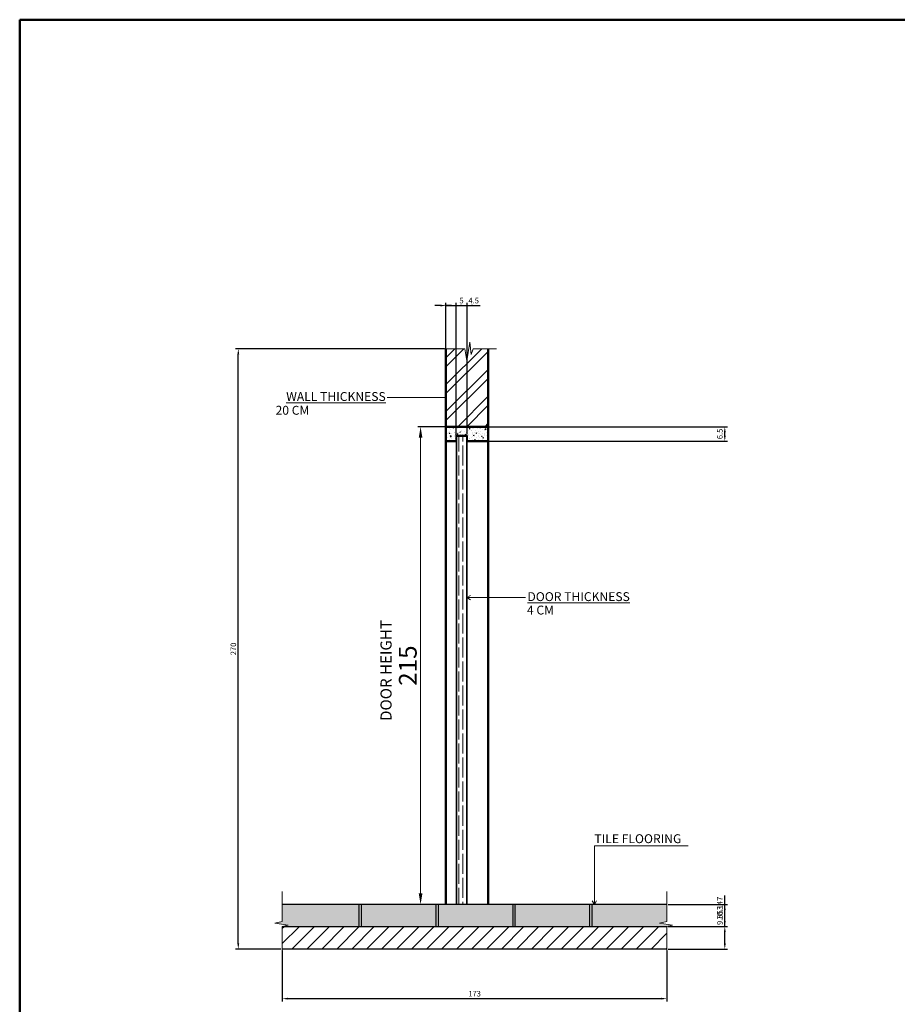
# Model space of a CAD drawing. Units: centimetres. Extents: x 1523 to 2760, y 1250 to 2134.
# Tile 2 of 4: x 1523 to 1918, y 1691 to 2134. Entities that reach past the tile are written whole.
import ezdxf

# ---------------------------------------------------------------- set-up
doc = ezdxf.new("R2010")
doc.units = ezdxf.units.CM
for name, color, linetype, lineweight in [('A-ANNO-DIMS', 2, 'Continuous', 18), ('A-ANNO-NPLT', 8, 'Continuous', 13), ('A-ANNO-SYMB', 7, 'Continuous', 18), ('A-ANNO-TEXT', 7, 'Continuous', 18), ('A-ANNO-TTLB', 7, 'Continuous', 50), ('A-DOOR', 4, 'Continuous', 35), ('A-DOOR-PATT', 251, 'Continuous', 13), ('A-FLOR', 7, 'Continuous', 25), ('A-FLOR-PATT', 251, 'Continuous', 13), ('A-WALL', 7, 'Continuous', 50), ('A-WALL-PATT', 251, 'Continuous', 13)]:
    doc.layers.add(name, color=color, linetype=linetype, lineweight=lineweight)
doc.styles.get("Standard").update_dxf_attribs({"font": 'arial.ttf'})
doc.dimstyles.new('ISO-25', dxfattribs={"dimtxt": 2.5, "dimasz": 2.5, "dimexe": 1.25, "dimexo": 0.625, "dimtad": 1, "dimtxsty": 'Standard', "dimcen": 2.5, "dimadec": 0, "dimazin": 0, "dimtfac": 1, "dimtmove": 0, "dimatfit": 3, "dimfxl": 1, "dimarcsym": 0})

# ---------------------------------------------------------------- blocks, each defined once
blk = doc.blocks.new('*D7')
at = {"layer": 'A-ANNO-DIMS', "color": 0, "lineweight": -2, "transparency": 16777216}
for p, q in [((1714.39, 1950.7), (1702.34, 1950.7)), ((1714.39, 1735.7), (1702.34, 1735.7))]:
    blk.add_line(p, q, dxfattribs=at)
at = {"layer": 'A-ANNO-DIMS', "color": 0, "lineweight": 0, "transparency": 16777216}
blk.add_line((1703.59, 1740.7), (1703.59, 1945.7), dxfattribs=at)
at = {"layer": 'A-ANNO-DIMS', "color": 0, "transparency": 16777216}
for points in [[(1702.76, 1945.7), (1704.42, 1945.7), (1703.59, 1950.7)], [(1702.76, 1740.7), (1704.42, 1740.7), (1703.59, 1735.7)]]:
    blk.add_solid(points, dxfattribs=at)
at = {"layer": 'Defpoints', "color": 0, "transparency": 16777216}
for p in [(1703.59, 1950.7), (1715.02, 1950.7), (1715.02, 1735.7)]:
    blk.add_point(p, dxfattribs=at)
at = {"layer": 'A-ANNO-DIMS', "color": 0, "transparency": 16777216, "insert": (1698.88, 1843.2), "char_height": 8, "width": 6.4304, "attachment_point": 5, "rotation": 90}
blk.add_mtext('215', dxfattribs=at)
blk = doc.blocks.new('BREAK-FLOOR')
for p, q in [((2.59, 31.69), (2.59, 18.28)), ((2.59, 18.28), (5.9, 17.46)), ((5.9, 17.46), (0, 16.6)), ((0, 16.6), (2.59, 15.97)), ((2.59, 15.97), (2.59, 0))]:
    blk.add_line(p, q)
blk = doc.blocks.new('LEADER-NOTE')
for q in [(1.66, 1.91), (26.45, 0.95), (1.66, 0)]:
    blk.add_line((0, 0.95), q)
blk = doc.blocks.new('BREAK-WALL-SECT')
for p, q in [((0, 5.33), (10.43, 5.33)), ((10.43, 5.33), (11.33, 2.85)), ((11.33, 2.85), (12, 8.33)), ((12, 8.33), (13.36, 0)), ((13.36, 0), (14.23, 5.33)), ((14.23, 5.33), (25.25, 5.33))]:
    blk.add_line(p, q)
blk = doc.blocks.new('*D36')
at = {"layer": 'A-ANNO-DIMS', "color": 0, "lineweight": -2, "transparency": 16777216}
for p, q in [((1641.39, 1715.08), (1641.39, 1692.13)), ((1814.39, 1715.08), (1814.39, 1692.13)), ((1643.89, 1693.38), (1811.89, 1693.38))]:
    blk.add_line(p, q, dxfattribs=at)
at = {"layer": 'A-ANNO-DIMS', "color": 0, "transparency": 16777216}
for points in [[(1643.89, 1693.8), (1643.89, 1692.97), (1641.39, 1693.38)], [(1811.89, 1693.8), (1811.89, 1692.97), (1814.39, 1693.38)]]:
    blk.add_solid(points, dxfattribs=at)
at = {"layer": 'Defpoints', "color": 0, "transparency": 16777216}
for p in [(1641.39, 1715.7), (1814.39, 1715.7), (1814.39, 1693.38)]:
    blk.add_point(p, dxfattribs=at)
at = {"layer": 'A-ANNO-DIMS', "color": 0, "transparency": 16777216, "insert": (1727.89, 1695.29), "char_height": 2.5, "attachment_point": 5}
blk.add_mtext('173', dxfattribs=at)
blk = doc.blocks.new('*D37')
at = {"layer": 'A-ANNO-DIMS', "color": 0, "lineweight": -2, "transparency": 16777216}
for p, q in [((1714.39, 1985.7), (1620.33, 1985.7)), ((1621.58, 1718.2), (1621.58, 1983.2)), ((1640.77, 1715.7), (1620.33, 1715.7))]:
    blk.add_line(p, q, dxfattribs=at)
at = {"layer": 'A-ANNO-DIMS', "color": 0, "transparency": 16777216}
for points in [[(1621.16, 1983.2), (1622, 1983.2), (1621.58, 1985.7)], [(1621.16, 1718.2), (1622, 1718.2), (1621.58, 1715.7)]]:
    blk.add_solid(points, dxfattribs=at)
at = {"layer": 'Defpoints', "color": 0, "transparency": 16777216}
for p in [(1621.58, 1985.7), (1715.02, 1985.7), (1641.39, 1715.7)]:
    blk.add_point(p, dxfattribs=at)
at = {"layer": 'A-ANNO-DIMS', "color": 0, "transparency": 16777216, "insert": (1619.68, 1850.7), "char_height": 2.5, "attachment_point": 5, "rotation": 90}
blk.add_mtext('270', dxfattribs=at)
blk = doc.blocks.new('*D38')
at = {"layer": 'A-ANNO-DIMS', "color": 0, "lineweight": -2, "transparency": 16777216}
for p, q in [((1734.64, 1950.7), (1841.69, 1950.7)), ((1840.44, 1946.7), (1840.44, 1948.2)), ((1734.64, 1944.2), (1841.69, 1944.2))]:
    blk.add_line(p, q, dxfattribs=at)
at = {"layer": 'A-ANNO-DIMS', "color": 0, "transparency": 16777216}
for points in [[(1840.03, 1948.2), (1840.86, 1948.2), (1840.44, 1950.7)], [(1840.03, 1946.7), (1840.86, 1946.7), (1840.44, 1944.2)]]:
    blk.add_solid(points, dxfattribs=at)
at = {"layer": 'Defpoints', "color": 0, "transparency": 16777216}
for p in [(1734.02, 1950.7), (1840.44, 1950.7), (1734.02, 1944.2)]:
    blk.add_point(p, dxfattribs=at)
at = {"layer": 'A-ANNO-DIMS', "color": 0, "transparency": 16777216, "insert": (1838.54, 1947.45), "char_height": 2.5, "attachment_point": 5, "rotation": 90}
blk.add_mtext('6.5', dxfattribs=at)
blk = doc.blocks.new('*D39')
at = {"layer": 'A-ANNO-DIMS', "color": 0, "lineweight": -2, "transparency": 16777216}
for p, q in [((1717.02, 2005.2), (1714.52, 2005.2)), ((1719.52, 1947.33), (1719.52, 2006.45)), ((1719.52, 2005.2), (1724.52, 2005.2)), ((1724.52, 1947.33), (1724.52, 2006.45)), ((1727.02, 2005.2), (1729.52, 2005.2))]:
    blk.add_line(p, q, dxfattribs=at)
at = {"layer": 'A-ANNO-DIMS', "color": 0, "transparency": 16777216}
for points in [[(1717.02, 2005.62), (1717.02, 2004.79), (1719.52, 2005.2)], [(1727.02, 2005.62), (1727.02, 2004.79), (1724.52, 2005.2)]]:
    blk.add_solid(points, dxfattribs=at)
at = {"layer": 'Defpoints', "color": 0, "transparency": 16777216}
for p in [(1724.52, 2005.2), (1719.52, 1946.7), (1724.52, 1946.7)]:
    blk.add_point(p, dxfattribs=at)
at = {"layer": 'A-ANNO-DIMS', "color": 0, "transparency": 16777216, "insert": (1722.02, 2007.1), "char_height": 2.5, "attachment_point": 5}
blk.add_mtext('5', dxfattribs=at)
blk = doc.blocks.new('*D40')
at = {"layer": 'A-ANNO-DIMS', "color": 0, "lineweight": -2, "transparency": 16777216}
for p, q in [((1712.52, 2005.2), (1710.02, 2005.2)), ((1715.02, 1944.83), (1715.02, 2006.45)), ((1715.02, 2005.2), (1719.52, 2005.2)), ((1719.52, 1944.83), (1719.52, 2006.45)), ((1722.02, 2005.2), (1730.44, 2005.2))]:
    blk.add_line(p, q, dxfattribs=at)
at = {"layer": 'A-ANNO-DIMS', "color": 0, "transparency": 16777216}
for points in [[(1712.52, 2005.62), (1712.52, 2004.79), (1715.02, 2005.2)], [(1722.02, 2005.62), (1722.02, 2004.79), (1719.52, 2005.2)]]:
    blk.add_solid(points, dxfattribs=at)
at = {"layer": 'Defpoints', "color": 0, "transparency": 16777216}
for p in [(1719.52, 2005.2), (1715.02, 1944.2), (1719.52, 1944.2)]:
    blk.add_point(p, dxfattribs=at)
at = {"layer": 'A-ANNO-DIMS', "color": 0, "transparency": 16777216, "insert": (1727.48, 2007.1), "char_height": 2.5, "attachment_point": 5}
blk.add_mtext('4.5', dxfattribs=at)
blk = doc.blocks.new('*D41')
at = {"layer": 'A-ANNO-DIMS', "color": 0, "lineweight": -2, "transparency": 16777216}
for p, q in [((1815.02, 1735.7), (1841.69, 1735.7)), ((1840.44, 1728.35), (1840.44, 1733.2)), ((1815.01, 1725.85), (1841.69, 1725.85))]:
    blk.add_line(p, q, dxfattribs=at)
at = {"layer": 'A-ANNO-DIMS', "color": 0, "transparency": 16777216}
for points in [[(1840.03, 1733.2), (1840.86, 1733.2), (1840.44, 1735.7)], [(1840.03, 1728.35), (1840.86, 1728.35), (1840.44, 1725.85)]]:
    blk.add_solid(points, dxfattribs=at)
at = {"layer": 'Defpoints', "color": 0, "transparency": 16777216}
for p in [(1814.39, 1735.7), (1840.44, 1735.7), (1814.38, 1725.85)]:
    blk.add_point(p, dxfattribs=at)
at = {"layer": 'A-ANNO-DIMS', "color": 0, "transparency": 16777216, "insert": (1838.54, 1730.78), "char_height": 2.5, "attachment_point": 5, "rotation": 90}
blk.add_mtext('9.853', dxfattribs=at)
blk = doc.blocks.new('*D42')
at = {"layer": 'A-ANNO-DIMS', "color": 0, "lineweight": -2, "transparency": 16777216}
for p, q in [((1840.44, 1725.85), (1840.44, 1739.74)), ((1815.01, 1725.85), (1841.69, 1725.85)), ((1840.44, 1718.2), (1840.44, 1723.35)), ((1815.02, 1715.7), (1841.69, 1715.7))]:
    blk.add_line(p, q, dxfattribs=at)
at = {"layer": 'A-ANNO-DIMS', "color": 0, "transparency": 16777216}
for points in [[(1840.03, 1723.35), (1840.86, 1723.35), (1840.44, 1725.85)], [(1840.03, 1718.2), (1840.86, 1718.2), (1840.44, 1715.7)]]:
    blk.add_solid(points, dxfattribs=at)
at = {"layer": 'Defpoints', "color": 0, "transparency": 16777216}
for p in [(1814.38, 1725.85), (1840.44, 1725.85), (1814.39, 1715.7)]:
    blk.add_point(p, dxfattribs=at)
at = {"layer": 'A-ANNO-DIMS', "color": 0, "transparency": 16777216, "insert": (1838.54, 1734.05), "char_height": 2.5, "attachment_point": 5, "rotation": 90}
blk.add_mtext('10.147', dxfattribs=at)

msp = doc.modelspace()

# ---------------------------------------------------------------- hatches: boundary and pattern name
at = {"layer": 'A-DOOR-PATT'}
h = msp.add_hatch(dxfattribs=at)
h.set_pattern_fill('AR-CONC', color=256, scale=0.02)
h.paths.add_polyline_path([(1734.02, 1950.7048), (1715.02, 1950.7048), (1715.02, 1944.2048), (1719.52, 1944.2048), (1719.52, 1946.7048), (1724.52, 1946.7048), (1724.52, 1944.2048), (1734.02, 1944.2048)])
h = msp.add_hatch(dxfattribs=at)
h.set_pattern_fill('GOST_WOOD', color=256, scale=0.9)
h.paths.add_polyline_path([(1724.32, 1946.5048), (1719.72, 1946.5048), (1719.72, 1945.7048), (1719.72, 1735.7048), (1724.32, 1735.7048)])
at = {"layer": 'A-FLOR-PATT'}
h = msp.add_hatch(dxfattribs=at)
h.set_pattern_fill('AR-CONC', color=256, scale=0.02)
h.paths.add_polyline_path([(1675.9881, 1735.7048), (1641.3937, 1735.7048), (1641.3937, 1728.1661), (1638.0785, 1727.3426), (1643.9809, 1726.4871), (1641.3875, 1725.8513), (1641.3875, 1725.7048), (1675.9881, 1725.7048)])
h.paths.add_polyline_path([(1710.5886, 1735.7048), (1676.9881, 1735.7048), (1676.9881, 1725.7048), (1710.5886, 1725.7048)])
h.paths.add_polyline_path([(1745.1892, 1735.7048), (1711.5886, 1735.7048), (1711.5886, 1725.7048), (1745.1892, 1725.7048)])
h.paths.add_polyline_path([(1779.7897, 1735.7048), (1746.1892, 1735.7048), (1746.1892, 1725.7048), (1779.7897, 1725.7048)])
h.paths.add_polyline_path([(1814.3902, 1735.7048), (1780.7897, 1735.7048), (1780.7897, 1725.7048), (1814.384, 1725.7048), (1814.384, 1725.8513), (1816.9774, 1726.4871), (1811.075, 1727.3426), (1814.3902, 1728.1661)])
h = msp.add_hatch(dxfattribs=at)
h.set_pattern_fill('ANSI31', color=256, scale=1.5)
h.set_pattern_definition([(45, (-599.5837, 298.8947), (-3.367596, 3.367596), [])])
h.paths.add_polyline_path([(1641.3875, 1725.7048), (1641.3903, 1715.7048), (1814.3868, 1715.7048), (1814.384, 1725.7048)])
at = {"layer": 'A-WALL-PATT'}
h = msp.add_hatch(dxfattribs=at)
h.set_pattern_fill('ANSI32', color=256, scale=0.9)
h.paths.add_polyline_path([(1734.02, 1985.7048), (1727.2839, 1985.7048), (1726.3782, 1983.2208), (1725.7123, 1988.7035), (1724.3538, 1980.373), (1723.482, 1985.7048), (1715.02, 1985.7048), (1715.02, 1950.7048), (1734.02, 1950.7048)])

# ---------------------------------------------------------------- linework, layer by layer
at = {"layer": 'A-ANNO-NPLT'}
for p in [(1675.9881, 1725.7048), (1710.5886, 1725.7048), (1745.1892, 1725.7048), (1779.7897, 1725.7048)]:
    msp.add_point(p, dxfattribs=at)
at = {"layer": 'A-ANNO-TEXT'}
for p, q in [((1715.02, 1963.8222), (1688.5687, 1963.8222)), ((1781.7664, 1735.7048), (1781.7664, 1762.1561)), ((1781.7664, 1762.1561), (1823.9421, 1762.1561)), ((1781.7664, 1735.7048), (1780.8118, 1737.3598)), ((1781.7664, 1735.7048), (1782.7209, 1737.3598))]:
    msp.add_line(p, q, dxfattribs=at)
at = {"layer": 'A-ANNO-TTLB'}
msp.add_lwpolyline([(1523.2447, 2133.8046), (2759.5532, 2133.8046), (2759.5532, 1250.2097), (1523.2447, 1250.2097)], close=True, dxfattribs=at)
at = {"layer": 'A-DOOR'}
for p, q in [((1724.52, 1946.7048), (1719.52, 1946.7048)), ((1719.52, 1946.7048), (1719.52, 1944.2048)), ((1719.72, 1735.7048), (1719.72, 1946.5048)), ((1724.32, 1946.5048), (1719.72, 1946.5048)), ((1719.72, 1946.5048), (1719.72, 1945.7048)), ((1724.32, 1735.7048), (1724.32, 1946.5048)), ((1724.32, 1945.7048), (1724.32, 1946.5048)), ((1724.52, 1944.2048), (1724.52, 1946.7048))]:
    msp.add_line(p, q, dxfattribs=at)
at = {"layer": 'A-FLOR'}
for p, q in [((1814.3902, 1735.7048), (1641.3937, 1735.7048)), ((1675.9881, 1725.7048), (1675.9881, 1735.7048)), ((1676.9881, 1725.7048), (1676.9881, 1735.7048)), ((1710.5886, 1725.7048), (1710.5886, 1735.7048)), ((1711.5886, 1725.7048), (1711.5886, 1735.7048)), ((1745.1892, 1725.7048), (1745.1892, 1735.7048)), ((1746.1892, 1725.7048), (1746.1892, 1735.7048)), ((1779.7897, 1725.7048), (1779.7897, 1735.7048)), ((1780.7897, 1725.7048), (1780.7897, 1735.7048)), ((1814.3902, 1725.7048), (1641.3875, 1725.7048)), ((1814.3902, 1715.7048), (1641.3903, 1715.7048))]:
    msp.add_line(p, q, dxfattribs=at)
at = {"layer": 'A-WALL'}
for p, q in [((1715.02, 1944.2048), (1715.02, 1985.7048)), ((1734.02, 1944.2048), (1734.02, 1985.7048)), ((1734.02, 1950.7048), (1715.02, 1950.7048)), ((1715.02, 1735.7048), (1715.02, 1945.7048)), ((1734.02, 1735.7048), (1734.02, 1945.7048)), ((1715.02, 1944.2048), (1719.52, 1944.2048)), ((1734.02, 1944.2048), (1724.52, 1944.2048))]:
    msp.add_line(p, q, dxfattribs=at)

# ---------------------------------------------------------------- block references
at = {"layer": 'A-ANNO-SYMB', "extrusion": (0, 0, -1), "zscale": -1}
for name, p in [('BREAK-WALL-SECT', (-1737.7127, 1980.3727)), ('BREAK-FLOOR', (-1643.9812, 1709.8837)), ('BREAK-FLOOR', (-1816.9777, 1709.8837))]:
    msp.add_blockref(name, p, dxfattribs=at)
at = {"layer": 'A-ANNO-TEXT'}
msp.add_blockref('LEADER-NOTE', (1724.3198, 1872.8464), dxfattribs=at)

# ---------------------------------------------------------------- texts
at = {"layer": 'A-ANNO-TEXT', "char_height": 4}
for s, insert, attachment_point in [('{\\fArial Rounded MT Bold|b0|i0|c0|p34;\\LWALL THICKNESS}', (1687.9067, 1966.2695), 3), ('{\\fArial Rounded MT Bold|b0|i0|c0|p34;20 CM}', (1638.3427, 1960.087), 1), ('{\\fArial Rounded MT Bold|b0|i0|c0|p34;\\LDOOR THICKNESS}', (1751.6624, 1876.2481), 1), ('{\\fArial Rounded MT Bold|b0|i0|c0|p34;4 CM}', (1751.4421, 1870.196), 1), ('{\\fArial Rounded MT Bold|b0|i0|c0|p34;TILE FLOORING}', (1781.7925, 1767.3401), 1)]:
    msp.add_mtext_dynamic_manual_height_columns(s, width=86.463106, gutter_width=12.5, heights=[0], dxfattribs=dict(at, insert=insert, attachment_point=attachment_point))
at = {"layer": 'A-ANNO-TEXT', "insert": (1690.5488, 1818.3116), "char_height": 5, "attachment_point": 7, "rotation": 90}
msp.add_mtext_dynamic_manual_height_columns('{\\fArial Rounded MT Bold|b0|i0|c0|p34;DOOR HEIGHT}', width=86.463106, gutter_width=12.5, heights=[0], dxfattribs=at)

# ---------------------------------------------------------------- dimensions: what is measured, and where the dimension line sits
at = {"layer": 'A-ANNO-DIMS'}
for base, p1, p2, override, picture, middle in [((1719.52, 2005.2035), (1715.02, 1944.2048), (1719.52, 1944.2048), {"dimdec": 1, "dimlfac": 1, "dimrnd": 0, "dimzin": 0, "dimdsep": 46, "dimlunit": 2}, '*D40', (1727.4804, 2007.0999)), ((1724.52, 2005.2035), (1719.52, 1946.7048), (1724.52, 1946.7048), {"dimdec": 0, "dimlfac": 1, "dimrnd": 0, "dimzin": 0, "dimdsep": 46, "dimlunit": 2}, '*D39', (1722.02, 2007.0999)), ((1814.3902, 1693.3841), (1641.3903, 1715.7048), (1814.3902, 1715.7048), {"dimdec": 0, "dimlfac": 1, "dimrnd": 0, "dimzin": 0, "dimdsep": 46, "dimlunit": 2}, '*D36', (1727.8903, 1695.2864))]:
    dim = msp.add_linear_dim(base=base, p1=p1, p2=p2, dimstyle='ISO-25', override=override, dxfattribs=at)
    dim.commit()
    dim.dimension.update_dxf_attribs({"geometry": picture, "text_midpoint": middle})
for base, p1, p2, override, picture, middle in [((1621.5785, 1985.7048), (1641.3903, 1715.7048), (1715.02, 1985.7048), {"dimdec": 0, "dimlfac": 1, "dimrnd": 0, "dimzin": 0, "dimdsep": 46, "dimlunit": 2}, '*D37', (1619.6771, 1850.7048)), ((1703.5916, 1950.7048), (1715.02, 1735.7048), (1715.02, 1950.7048), {"dimtxt": 8, "dimasz": 5, "dimclrd": 0, "dimclre": 0, "dimclrt": 0, "dimlwd": 0}, '*D7', (1698.882, 1843.2048)), ((1840.4421, 1950.7048), (1734.02, 1944.2048), (1734.02, 1950.7048), {"dimdec": 1, "dimlfac": 1, "dimrnd": 0, "dimzin": 0, "dimdsep": 46, "dimlunit": 2}, '*D38', (1838.5406, 1947.4548)), ((1840.44206, 1725.85133), (1814.39024, 1715.70479), (1814.38399, 1725.85133), {"dimdec": 3, "dimlfac": 1, "dimrnd": 0, "dimzin": 0, "dimdsep": 46, "dimlunit": 2}, '*D42', (1838.54062, 1734.04796)), ((1840.44206, 1735.70479), (1814.38399, 1725.85133), (1814.39024, 1735.70479), {"dimdec": 3, "dimlfac": 1, "dimrnd": 0, "dimzin": 0, "dimdsep": 46, "dimlunit": 2}, '*D41', (1838.53977, 1730.77806))]:
    dim = msp.add_linear_dim(base=base, p1=p1, p2=p2, angle=90, dimstyle='ISO-25', override=override, dxfattribs=at)
    dim.commit()
    dim.dimension.update_dxf_attribs({"geometry": picture, "text_midpoint": middle})

doc.saveas('drawing.dxf')
